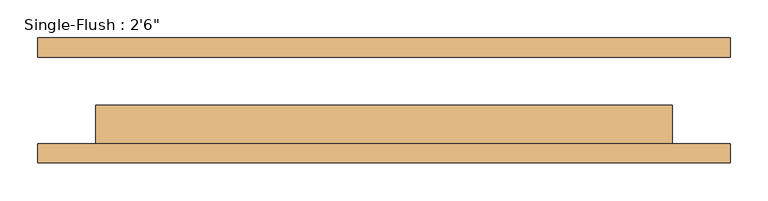
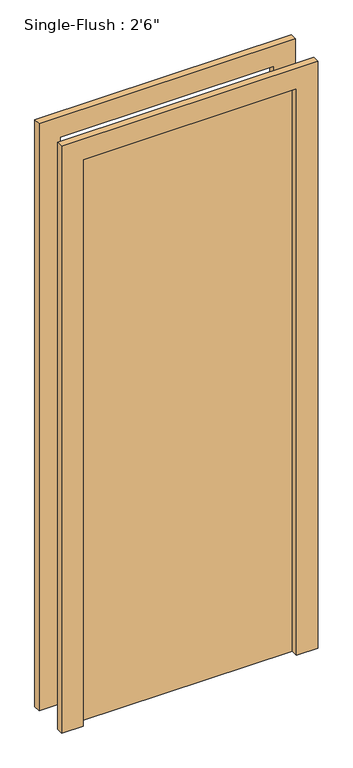
"""IFC4 building model written with IfcOpenShell, lengths in millimetres: door geometry."""

from ifc_helpers import new_model, si_unit, frame, origin, origin_with_axes, place, context, project, spatial, polyline, outline, extrude, source, transform, mapped, element, save


def door_78caadf7(model_context):
    return source(origin(), model_context, "Body", "SweptSolid", [
        extrude(outline(polyline([(2209.8, -457.2), (0.0, -457.2), (0.0, -381.0), (2133.6, -381.0), (2133.6, 381.0), (0.0, 381.0), (0.0, 457.2), (2209.8, 457.2), (2209.8, -457.2)])), frame((0.0, -82.55, 0.0), z_axis=(0.0, 1.0, 0.0), x_axis=(0.0, 0.0, 1.0)), (0.0, 0.0, 1.0), 25.4),
        extrude(outline(polyline([(2209.8, 457.2), (2209.8, -457.2), (0.0, -457.2), (0.0, -381.0), (2133.6, -381.0), (2133.6, 381.0), (0.0, 381.0), (0.0, 457.2), (2209.8, 457.2)])), frame((0.0, 57.15, 0.0), z_axis=(0.0, 1.0, 0.0), x_axis=(0.0, 0.0, 1.0)), (0.0, 0.0, 1.0), 25.4),
        extrude(outline(polyline([(381.0, -6.35), (381.0, -57.15), (-381.0, -57.15), (-381.0, -6.35), (381.0, -6.35)])), origin_with_axes(), (0.0, 0.0, 1.0), 2133.6),
    ])


if __name__ == "__main__":
    model = new_model("IFC4")
    model_context = context("Model", 3, world=origin())
    ifc_project = project(units=[si_unit("LENGTHUNIT", "METRE", prefix="MILLI")], contexts=[model_context])
    site = spatial("IfcSite", under=ifc_project)
    building = spatial("IfcBuilding", under=site)
    placement = place(None, origin())
    door_shape = door_78caadf7(model_context)
    element("IfcDoor", 1, ObjectType="Single-Flush : 2'6\"", at=placement, inside=building, context=model_context, shape_type="MappedRepresentation", body=[
        mapped(door_shape, transform((0.0, 0.0, 0.0), x_axis=(1.0, 0.0, 0.0), y_axis=(0.0, 1.0, 0.0), z_axis=(0.0, 0.0, 1.0))),
    ])
    save(model, "model.ifc")

# Revit data of these elements
# Type "Single-Flush : 2'6\""
#   Type Mark = "9"
#   Construction Type Id = "MDOOR"
#   Assembly Code = "C1020"
#   Analytic Construction = "Metal"
#   Thickness = 0' - 2"
#   Heat Transfer Coefficient (U) = 0.651978 BTU/(h·ft²·°F)
#   Height = 7' - 0"
#   Trim Projection Ext = 0' - 1"
#   Trim Projection Int = 0' - 1"
#   Trim Width = 0' - 3"
#   Width = 2' - 6"
#   Define Thermal Properties by = 1
#   Door Material = Door - Panel
#   Frame Material = Door - Frame
#   Visual Light Transmittance = 0
#   Solar Heat Gain Coefficient = 0
#   Function = (empty or 0)
#   Wall Closure = (empty or 0)
# Element 1 (IfcDoor, "Single-Flush : 2'6\"")
#   Materials on its faces: "Door - Frame", "Door - Panel"
# Materials
#   "Door - Panel": class "Wood", colour RGB 210 159 95, transparency 0, Cost = 0
#   "Door - Frame": colour RGB 118 70 51, transparency 0, Cost = 0
